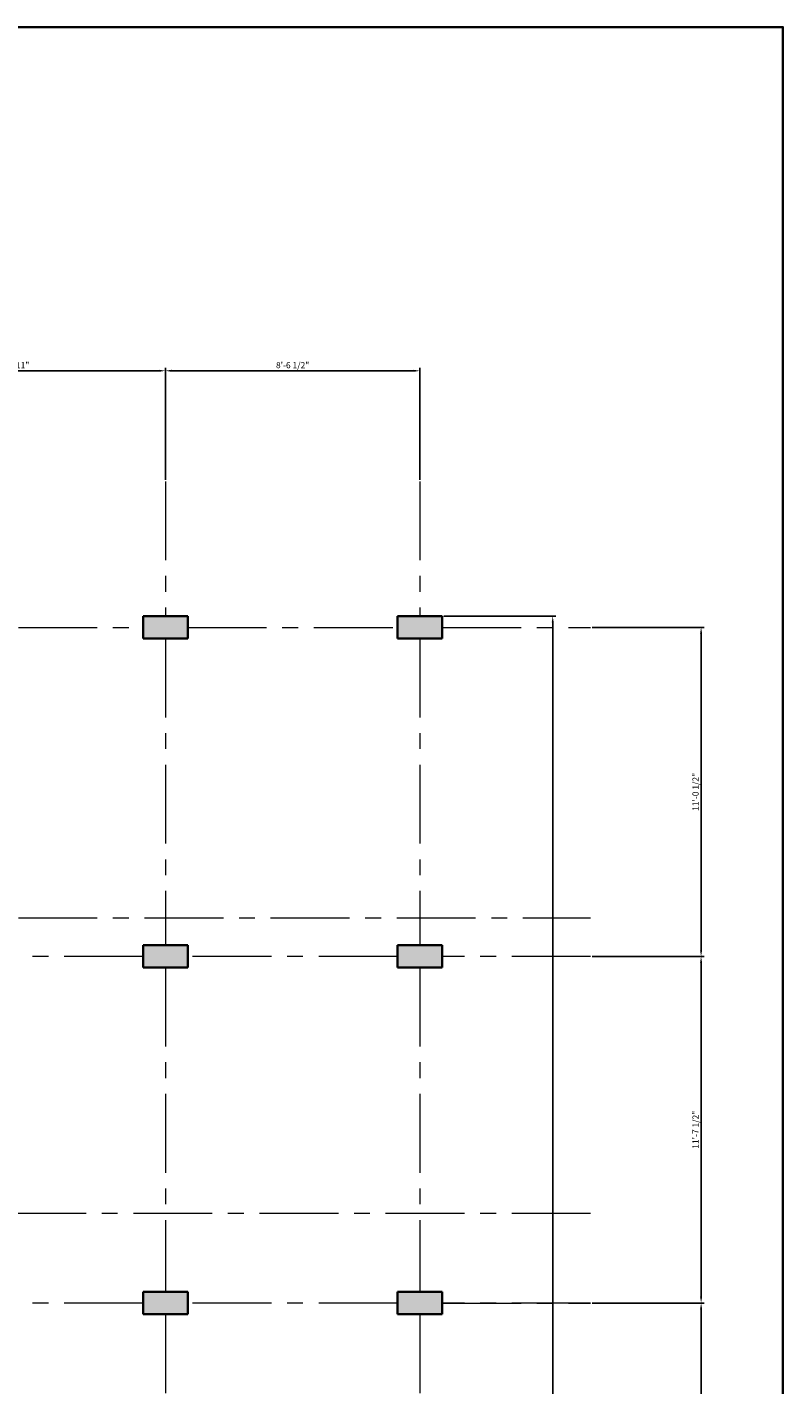
# Model space of a CAD drawing. Units: inches. Extents: x 2391 to 16591, y 7259 to 10239.
# Tile 25 of 27: x 3850 to 4154, y 9693 to 10239. Entities that reach past the tile are written whole.
import ezdxf

# ---------------------------------------------------------------- set-up
doc = ezdxf.new("R2010")
doc.units = ezdxf.units.IN
doc.linetypes.add('CENTER', pattern=[50.8, 31.75, -6.35, 6.35, -6.35])
for name, color, linetype, lineweight in [('A-ANNO-DIMS', 4, 'Continuous', 18), ('A-ANNO-TTLB', 7, 'Continuous', 35), ('A-COLS', 3, 'Continuous', 35), ('A-COLS-PATT', 3, 'Continuous', 13), ('A-GRID', 1, 'CENTER', 13)]:
    doc.layers.add(name, color=color, linetype=linetype, lineweight=lineweight)
doc.styles.get("Standard").update_dxf_attribs({"font": 'arial.ttf'})
doc.dimstyles.new('ISO-25', dxfattribs={"dimtxt": 2.5, "dimasz": 2.5, "dimexe": 1.25, "dimexo": 0.625, "dimtad": 1, "dimdec": 0, "dimlunit": 3, "dimtxsty": 'Standard', "dimcen": 2.5, "dimadec": 0, "dimazin": 0, "dimtfac": 1, "dimtdec": 0, "dimtmove": 0, "dimatfit": 3, "dimfxl": 1, "dimarcsym": 0})

# ---------------------------------------------------------------- blocks, each defined once
blk = doc.blocks.new('*D103')
at = {"layer": 'A-ANNO-DIMS', "color": 0, "lineweight": -2, "transparency": 16777216}
for p, q in [((4017.64, 10002.26), (4062.76, 10002.26)), ((4061.51, 9999.76), (4061.51, 9356.76)), ((4017.64, 9354.26), (4062.76, 9354.26))]:
    blk.add_line(p, q, dxfattribs=at)
at = {"layer": 'A-ANNO-DIMS', "color": 0, "transparency": 16777216}
for points in [[(4061.1, 9999.76), (4061.93, 9999.76), (4061.51, 10002.26)], [(4061.1, 9356.76), (4061.93, 9356.76), (4061.51, 9354.26)]]:
    blk.add_solid(points, dxfattribs=at)
at = {"layer": 'Defpoints', "color": 0, "transparency": 16777216}
for p in [(4017.01, 10002.26), (4017.01, 9354.26), (4061.51, 9354.26)]:
    blk.add_point(p, dxfattribs=at)
at = {"layer": 'A-ANNO-DIMS', "color": 0, "transparency": 16777216, "insert": (4059.61, 9678.26), "char_height": 2.5, "attachment_point": 5, "rotation": 90}
blk.add_mtext('54\'-0"', dxfattribs=at)
blk = doc.blocks.new('*D105')
at = {"layer": 'A-ANNO-DIMS', "color": 0, "lineweight": -2, "transparency": 16777216}
for p, q in [((3786.51, 10057.17), (3786.51, 10102.29)), ((3789.01, 10101.04), (3903.01, 10101.04)), ((3905.51, 10057.17), (3905.51, 10102.29))]:
    blk.add_line(p, q, dxfattribs=at)
at = {"layer": 'A-ANNO-DIMS', "color": 0, "transparency": 16777216}
for points in [[(3789.01, 10101.46), (3789.01, 10100.63), (3786.51, 10101.04)], [(3903.01, 10101.46), (3903.01, 10100.63), (3905.51, 10101.04)]]:
    blk.add_solid(points, dxfattribs=at)
at = {"layer": 'Defpoints', "color": 0, "transparency": 16777216}
for p in [(3905.51, 10101.04), (3786.51, 10056.54), (3905.51, 10056.54)]:
    blk.add_point(p, dxfattribs=at)
at = {"layer": 'A-ANNO-DIMS', "color": 0, "transparency": 16777216, "insert": (3846.01, 10102.95), "char_height": 2.5, "attachment_point": 5}
blk.add_mtext('9\'-11"', dxfattribs=at)
blk = doc.blocks.new('*D106')
at = {"layer": 'A-ANNO-DIMS', "color": 0, "lineweight": -2, "transparency": 16777216}
for p, q in [((3905.51, 10057.17), (3905.51, 10102.29)), ((3908.01, 10101.04), (4005.51, 10101.04)), ((4008.01, 10057.17), (4008.01, 10102.29))]:
    blk.add_line(p, q, dxfattribs=at)
at = {"layer": 'A-ANNO-DIMS', "color": 0, "transparency": 16777216}
for points in [[(3908.01, 10101.46), (3908.01, 10100.63), (3905.51, 10101.04)], [(4005.51, 10101.46), (4005.51, 10100.63), (4008.01, 10101.04)]]:
    blk.add_solid(points, dxfattribs=at)
at = {"layer": 'Defpoints', "color": 0, "transparency": 16777216}
for p in [(4008.01, 10101.04), (3905.51, 10056.54), (4008.01, 10056.54)]:
    blk.add_point(p, dxfattribs=at)
at = {"layer": 'A-ANNO-DIMS', "color": 0, "transparency": 16777216, "insert": (3956.76, 10102.96), "char_height": 2.5, "attachment_point": 5}
blk.add_mtext('8\'-6 1/2"', dxfattribs=at)
blk = doc.blocks.new('*D114')
at = {"layer": 'A-ANNO-DIMS', "color": 0, "lineweight": -2, "transparency": 16777216}
for p, q in [((4077.4, 9725.76), (4122.52, 9725.76)), ((4121.27, 9639.26), (4121.27, 9723.26)), ((4077.4, 9636.76), (4122.52, 9636.76))]:
    blk.add_line(p, q, dxfattribs=at)
at = {"layer": 'A-ANNO-DIMS', "color": 0, "transparency": 16777216}
for points in [[(4120.86, 9723.26), (4121.69, 9723.26), (4121.27, 9725.76)], [(4120.86, 9639.26), (4121.69, 9639.26), (4121.27, 9636.76)]]:
    blk.add_solid(points, dxfattribs=at)
at = {"layer": 'Defpoints', "color": 0, "transparency": 16777216}
for p in [(4076.77, 9725.76), (4121.27, 9725.76), (4076.77, 9636.76)]:
    blk.add_point(p, dxfattribs=at)
at = {"layer": 'A-ANNO-DIMS', "color": 0, "transparency": 16777216, "insert": (4119.38, 9681.26), "char_height": 2.5, "attachment_point": 5, "rotation": 90}
blk.add_mtext('7\'-5"', dxfattribs=at)
blk = doc.blocks.new('*D115')
at = {"layer": 'A-ANNO-DIMS', "color": 0, "lineweight": -2, "transparency": 16777216}
for p, q in [((4077.4, 9865.26), (4122.52, 9865.26)), ((4121.27, 9728.26), (4121.27, 9862.76)), ((4077.4, 9725.76), (4122.52, 9725.76))]:
    blk.add_line(p, q, dxfattribs=at)
at = {"layer": 'A-ANNO-DIMS', "color": 0, "transparency": 16777216}
for points in [[(4120.86, 9862.76), (4121.69, 9862.76), (4121.27, 9865.26)], [(4120.86, 9728.26), (4121.69, 9728.26), (4121.27, 9725.76)]]:
    blk.add_solid(points, dxfattribs=at)
at = {"layer": 'Defpoints', "color": 0, "transparency": 16777216}
for p in [(4076.77, 9865.26), (4121.27, 9865.26), (4076.77, 9725.76)]:
    blk.add_point(p, dxfattribs=at)
at = {"layer": 'A-ANNO-DIMS', "color": 0, "transparency": 16777216, "insert": (4119.36, 9795.51), "char_height": 2.5, "attachment_point": 5, "rotation": 90}
blk.add_mtext('11\'-7 1/2"', dxfattribs=at)
blk = doc.blocks.new('*D116')
at = {"layer": 'A-ANNO-DIMS', "color": 0, "lineweight": -2, "transparency": 16777216}
for p, q in [((4077.4, 9997.76), (4122.52, 9997.76)), ((4121.27, 9867.76), (4121.27, 9995.26)), ((4077.4, 9865.26), (4122.52, 9865.26))]:
    blk.add_line(p, q, dxfattribs=at)
at = {"layer": 'A-ANNO-DIMS', "color": 0, "transparency": 16777216}
for points in [[(4120.86, 9995.26), (4121.69, 9995.26), (4121.27, 9997.76)], [(4120.86, 9867.76), (4121.69, 9867.76), (4121.27, 9865.26)]]:
    blk.add_solid(points, dxfattribs=at)
at = {"layer": 'Defpoints', "color": 0, "transparency": 16777216}
for p in [(4076.77, 9997.76), (4121.27, 9997.76), (4076.77, 9865.26)]:
    blk.add_point(p, dxfattribs=at)
at = {"layer": 'A-ANNO-DIMS', "color": 0, "transparency": 16777216, "insert": (4119.36, 9931.51), "char_height": 2.5, "attachment_point": 5, "rotation": 90}
blk.add_mtext('11\'-0 1/2"', dxfattribs=at)

msp = doc.modelspace()

# ---------------------------------------------------------------- hatches: boundary and pattern name
at = {"layer": 'A-COLS-PATT'}
h = msp.add_hatch(color=256, dxfattribs=at)
h.dxf.hatch_style = 1
h.paths.add_polyline_path([(3674.26, 9993.26), (3674.26, 10002.26), (3656.26, 10002.26), (3656.26, 9993.26)])
h.paths.add_polyline_path([(3777.51, 10002.26), (3777.51, 9993.26), (3795.51, 9993.26), (3795.51, 10002.26)])
h.paths.add_polyline_path([(3896.51, 10002.26), (3896.51, 9993.26), (3914.51, 9993.26), (3914.51, 10002.26)])
h.paths.add_polyline_path([(3999.01, 10002.26), (3999.01, 9993.26), (4017.01, 9993.26), (4017.01, 10002.26)])
h.paths.add_polyline_path([(4017.01, 9860.76), (4017.01, 9869.76), (3999.01, 9869.76), (3999.01, 9860.76)])
h.paths.add_polyline_path([(3914.51, 9860.76), (3914.51, 9869.76), (3896.51, 9869.76), (3896.51, 9860.76)])
h.paths.add_polyline_path([(3777.51, 9885.26), (3777.51, 9876.26), (3795.51, 9876.26), (3795.51, 9885.26)])
h.paths.add_polyline_path([(3674.26, 9876.26), (3674.26, 9885.26), (3656.26, 9885.26), (3656.26, 9876.26)])
h.paths.add_polyline_path([(3656.26, 9766.26), (3656.26, 9757.26), (3674.26, 9757.26), (3674.26, 9766.26)])
h.paths.add_polyline_path([(3786.51, 9759.76), (3795.51, 9759.76), (3795.51, 9777.76), (3786.51, 9777.76)])
h.paths.add_polyline_path([(3914.51, 9721.26), (3914.51, 9730.26), (3896.51, 9730.26), (3896.51, 9721.26)])
h.paths.add_polyline_path([(3999.01, 9730.26), (3999.01, 9721.26), (4017.01, 9721.26), (4017.01, 9730.26)])
h.paths.add_polyline_path([(4017.01, 9632.26), (4017.01, 9641.26), (3999.01, 9641.26), (3999.01, 9632.26)])
h.paths.add_polyline_path([(3914.51, 9632.26), (3914.51, 9641.26), (3896.51, 9641.26), (3896.51, 9632.26)])
h.paths.add_polyline_path([(3795.51, 9632.26), (3786.51, 9632.26), (3786.51, 9614.26), (3795.51, 9614.26)])
h.paths.add_polyline_path([(3656.26, 9602.26), (3656.26, 9593.26), (3674.26, 9593.26), (3674.26, 9602.26)])
h.paths.add_polyline_path([(3674.26, 9471.26), (3674.26, 9480.26), (3656.26, 9480.26), (3656.26, 9471.26)])
h.paths.add_polyline_path([(3795.51, 9489.26), (3786.51, 9489.26), (3786.51, 9471.26), (3795.51, 9471.26)])
h.paths.add_polyline_path([(3896.51, 9502.76), (3896.51, 9493.76), (3914.51, 9493.76), (3914.51, 9502.76)])
h.paths.add_polyline_path([(3999.01, 9502.76), (3999.01, 9493.76), (4017.01, 9493.76), (4017.01, 9502.76)])
h.paths.add_polyline_path([(4017.01, 9354.26), (4017.01, 9363.26), (3999.01, 9363.26), (3999.01, 9354.26)])
h.paths.add_polyline_path([(3914.51, 9354.26), (3914.51, 9363.26), (3896.51, 9363.26), (3896.51, 9354.26)])
h.paths.add_polyline_path([(3795.51, 9354.26), (3795.51, 9363.26), (3777.51, 9363.26), (3777.51, 9354.26)])
h.paths.add_polyline_path([(3674.26, 9354.26), (3674.26, 9363.26), (3656.26, 9363.26), (3656.26, 9354.26)])

# ---------------------------------------------------------------- linework, layer by layer
at = {"layer": 'A-ANNO-TTLB'}
msp.add_lwpolyline([(2391.28, 10239.38), (4154.2, 10239.38), (4154.2, 7258.54), (2391.28, 7258.54)], close=True, dxfattribs=at)
at = {"layer": 'A-COLS'}
for p, q in [((3896.51, 10002.26), (3914.51, 10002.26)), ((3896.51, 9993.26), (3896.51, 10002.26)), ((3914.51, 10002.26), (3914.51, 9993.26)), ((3999.01, 10002.26), (4017.01, 10002.26)), ((3999.01, 9993.26), (3999.01, 10002.26)), ((4017.01, 10002.26), (4017.01, 9993.26)), ((3914.51, 9993.26), (3896.51, 9993.26)), ((4017.01, 9993.26), (3999.01, 9993.26)), ((3896.51, 9869.76), (3914.51, 9869.76)), ((3896.51, 9860.76), (3896.51, 9869.76)), ((3914.51, 9869.76), (3914.51, 9860.76)), ((3999.01, 9869.76), (4017.01, 9869.76)), ((3999.01, 9860.76), (3999.01, 9869.76)), ((4017.01, 9869.76), (4017.01, 9860.76)), ((3914.51, 9860.76), (3896.51, 9860.76)), ((4017.01, 9860.76), (3999.01, 9860.76)), ((3896.51, 9730.26), (3914.51, 9730.26)), ((3896.51, 9721.26), (3896.51, 9730.26)), ((3914.51, 9730.26), (3914.51, 9721.26)), ((3999.01, 9730.26), (4017.01, 9730.26)), ((3999.01, 9721.26), (3999.01, 9730.26)), ((4017.01, 9730.26), (4017.01, 9721.26)), ((3914.51, 9721.26), (3896.51, 9721.26)), ((4017.01, 9721.26), (3999.01, 9721.26))]:
    msp.add_line(p, q, dxfattribs=at)
at = {"layer": 'A-GRID'}
for p, q in [((3905.51, 10056.54), (3905.51, 10002.26)), ((4008.01, 10056.54), (4008.01, 10002.26)), ((3795.51, 9997.76), (3896.51, 9997.76)), ((3914.51, 9997.76), (3999.01, 9997.76)), ((4017.01, 9997.76), (4076.77, 9997.76)), ((3905.51, 9993.26), (3905.51, 9869.76)), ((4008.01, 9993.26), (4008.01, 9869.76)), ((3795.51, 9880.76), (4076.77, 9880.76)), ((4017.01, 9863.26), (4017.01, 9867.26)), ((3896.51, 9865.26), (3602.07, 9865.26)), ((3905.51, 9860.76), (3905.51, 9730.26)), ((3999.01, 9865.26), (3914.51, 9865.26)), ((4008.01, 9860.76), (4008.01, 9730.26)), ((4076.77, 9865.26), (4017.01, 9865.26)), ((4076.77, 9761.76), (3795.51, 9761.76)), ((3896.51, 9725.76), (3602.07, 9725.76)), ((3999.01, 9725.76), (3914.51, 9725.76)), ((4076.77, 9725.76), (4017.01, 9725.76)), ((4017.01, 9725.76), (4076.77, 9725.76)), ((3905.51, 9721.26), (3905.51, 9641.26)), ((4008.01, 9721.26), (4008.01, 9641.26))]:
    msp.add_line(p, q, dxfattribs=at)

# ---------------------------------------------------------------- dimensions: what is measured, and where the dimension line sits
at = {"layer": 'A-ANNO-DIMS'}
for base, p1, p2, picture, middle in [((4008.01, 10101.04), (3905.51, 10056.54), (4008.01, 10056.54), '*D106', (3956.76, 10102.96)), ((3905.51, 10101.04), (3786.51, 10056.54), (3905.51, 10056.54), '*D105', (3846.01, 10102.95))]:
    dim = msp.add_linear_dim(base=base, p1=p1, p2=p2, dimstyle='ISO-25', override={"dimdec": 1, "dimlfac": 1, "dimrnd": 0, "dimzin": 1, "dimdsep": 46, "dimlunit": 4, "dimfrac": 2}, dxfattribs=at)
    dim.commit()
    dim.dimension.update_dxf_attribs({"geometry": picture, "text_midpoint": middle})
for base, p1, p2, angle, picture, middle in [((4061.51, 9354.26), (4017.01, 10002.26), (4017.01, 9354.26), 270, '*D103', (4059.61, 9678.26)), ((4121.27, 9997.76), (4076.77, 9865.26), (4076.77, 9997.76), 90, '*D116', (4119.36, 9931.51)), ((4121.27, 9865.26), (4076.77, 9725.76), (4076.77, 9865.26), 90, '*D115', (4119.36, 9795.51)), ((4121.27, 9725.76), (4076.77, 9636.76), (4076.77, 9725.76), 90, '*D114', (4119.38, 9681.26))]:
    dim = msp.add_linear_dim(base=base, p1=p1, p2=p2, angle=angle, dimstyle='ISO-25', override={"dimdec": 1, "dimlfac": 1, "dimrnd": 0, "dimzin": 1, "dimdsep": 46, "dimlunit": 4, "dimfrac": 2}, dxfattribs=at)
    dim.commit()
    dim.dimension.update_dxf_attribs({"geometry": picture, "text_midpoint": middle})

doc.saveas('drawing.dxf')
